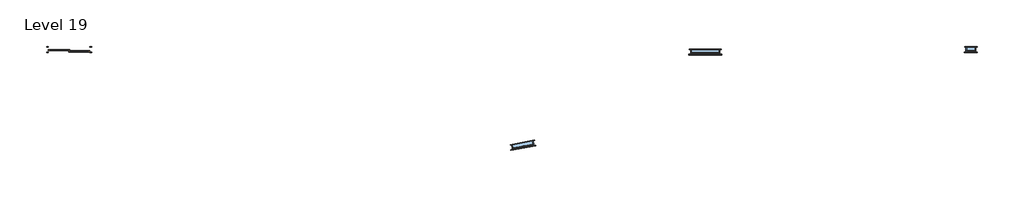
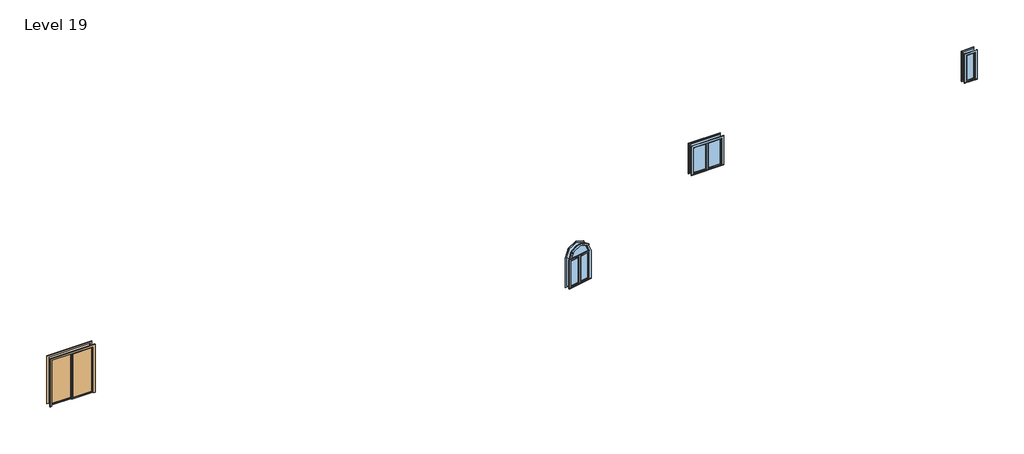
# One storey: 3 windows, 1 door.
"""IFC4 building model written with IfcOpenShell, lengths in millimetres."""

from ifc_helpers import new_model, si_unit, origin, place, context, project, spatial, transform, mapped, element, save
from components import door_076b30e0, window_cf4adaea, window_a765b88f, window_0862ab64

model = new_model("IFC4")

# Units and contexts
model_context = context("Model", 3, world=origin())
ifc_project = project(units=[si_unit("LENGTHUNIT", "METRE", prefix="MILLI")], contexts=[model_context])

# Site, building, storey
site = spatial("IfcSite", under=ifc_project)
building = spatial("IfcBuilding", under=site)
storey = spatial("IfcBuildingStorey", under=building, Name="Level 19", Elevation=32918.4)

# Door
placement = place(None, origin())
door_shape = door_076b30e0(model_context)
element("IfcDoor", 1, ObjectType="Door-Double-Sliding : 68\" x 80\"", at=placement, inside=storey, context=model_context, shape_type="MappedRepresentation", body=[
    mapped(door_shape, transform((-16521.785279, -12227.7237084, 32918.4), x_axis=(-1.0, 0.0, 0.0), y_axis=(0.0, -1.0, 0.0), z_axis=(0.0, 0.0, 1.0))),
])

# Windows
window_shape = window_cf4adaea(model_context)
element("IfcWindow", 2, ObjectType="36\" x 48\"", at=placement, inside=storey, context=model_context, shape_type="MappedRepresentation", body=[
    mapped(window_shape, transform((2348.7105307, -16344.9215105, 32918.4), x_axis=(-0.9830283621128597, -0.1834536434135567, 0.0), y_axis=(0.1834536434135567, -0.9830283621128597, 0.0), z_axis=(0.0, 0.0, 1.0))),
])
window_2_shape = window_a765b88f(model_context)
element("IfcWindow", 3, ObjectType="Awning with Trim : 16\" x 48\"", at=placement, inside=storey, context=model_context, shape_type="MappedRepresentation", body=[
    mapped(window_2_shape, transform((20968.614721, -12354.7237084, 32918.4), x_axis=(-1.0, 0.0, 0.0), y_axis=(0.0, -1.0, 0.0), z_axis=(0.0, 0.0, 1.0))),
])
window_3_shape = window_0862ab64(model_context)
element("IfcWindow", 4, ObjectType="Casement Dbl with Trim : 48\" x 48\"", at=placement, inside=storey, context=model_context, shape_type="MappedRepresentation", body=[
    mapped(window_3_shape, transform((9924.3594464, -12437.2737084, 32918.4), x_axis=(-1.0, 0.0, 0.0), y_axis=(0.0, -1.0, 0.0), z_axis=(0.0, 0.0, 1.0))),
])

save(model, "model.ifc")

# Revit data of these elements
# Type "Door-Double-Sliding : 68\" x 80\""
#   Type Mark = "10"
#   Construction Type Id = "opn-d45"
#   Assembly Code = "C1020"
#   Analytic Construction = "Wood frame, double glass door "
#   Thickness = 0' - 2"
#   Thermal Resistance (R) = 1.8150 (h·ft²·°F)/BTU
#   Heat Transfer Coefficient (U) = 0.5510 BTU/(h·ft²·°F)
#   Height = 6' - 8"
#   Rail Width = 0' - 2"
#   Stiles = 0' - 2"
#   Trim Projection Ext = 0' - 1"
#   Trim Projection Int = 0' - 1"
#   Trim Width = 0' - 3"
#   Width = 5' - 8"
#   Define Thermal Properties by = 1
#   Glazing = Glass
#   Panel Material = Wood - Birch - Solid Stained Light Low Gloss
#   Trim Material = Paint - Sienna
#   Visual Light Transmittance = 0
#   Solar Heat Gain Coefficient = 0
#   Function = (empty or 0)
#   Wall Closure = (empty or 0)
# Type "36\" x 48\""
#   Type Mark = "38"
#   Construction Type Id = "SGL"
#   Assembly Code = "B2020100"
#   Analytic Construction = "Large single-glazed windows"
#   Visual Light Transmittance = 0.9
#   Solar Heat Gain Coefficient = 0.86
#   Heat Transfer Coefficient (U) = 0.979472 BTU/(h·ft²·°F)
#   Height = 4' - 0"
#   Default Sill Height = 3' - 0"
#   Trim Projection - Ext. = 0' - 0 1/2"
#   Trim Projection - Int. = 0' - 0 3/4"
#   Trim Width - Exterior = 0' - 3 1/2"
#   Trim Width - Interior = 0' - 3 1/2"
#   Width = 3' - 0"
#   Window Inset = 0' - 0 3/4"
#   Define Thermal Properties by = 1
#   Glass Pane Material = Glass
#   Sash Material = Sash
#   Trim Exterior Material = Trim
#   Trim Interior Material = Trim
#   Wall Closure = (empty or 0)
# Type "Awning with Trim : 16\" x 48\""
#   Type Mark = "14"
#   Construction Type Id = "GSP4R"
#   Assembly Code = "B2020100"
#   Analytic Construction = "1/8 in Pilkington single glazing"
#   Visual Light Transmittance = 0.9
#   Solar Heat Gain Coefficient = 0.78
#   Heat Transfer Coefficient (U) = 0.6496 BTU/(h·ft²·°F)
#   Height = 4' - 0"
#   Default Sill Height = 3' - 0"
#   Trim Projection - Ext. = 0' - 0 1/2"
#   Trim Projection - Int. = 0' - 0 3/4"
#   Trim Width - Exterior = 0' - 3 1/2"
#   Trim Width - Interior = 0' - 3 1/2"
#   Width = 1' - 4"
#   Window Inset = 0' - 0 3/4"
#   Define Thermal Properties by = 1
#   Glass Pane Material = Glass
#   Sash Material = Sash
#   Trim Exterior Material = Trim
#   Trim Interior Material = Trim
#   Wall Closure = (empty or 0)
# Type "Casement Dbl with Trim : 48\" x 48\""
#   Type Mark = "34"
#   Construction Type Id = "GSP4R"
#   Assembly Code = "B2020100"
#   Analytic Construction = "1/8 in Pilkington single glazing"
#   Visual Light Transmittance = 0.9
#   Solar Heat Gain Coefficient = 0.78
#   Heat Transfer Coefficient (U) = 0.6496 BTU/(h·ft²·°F)
#   Height = 4' - 0"
#   Default Sill Height = 3' - 0"
#   Trim Projection - Ext. = 0' - 0 1/2"
#   Trim Projection - Int. = 0' - 0 3/4"
#   Trim Width - Exterior = 0' - 3 1/2"
#   Trim Width - Interior = 0' - 3 1/2"
#   Width = 4' - 0"
#   Window Inset = 0' - 0 3/4"
#   Define Thermal Properties by = 1
#   Glass Pane Material = Glass
#   Sash Material = Sash
#   Trim Exterior Material = Trim
#   Trim Interior Material = Trim
#   Wall Closure = (empty or 0)
# Element 1 (IfcDoor, "Door-Double-Sliding : 68\" x 80\"")
#   Phase Created = New Construction
#   Materials on its faces: "Paint - Sienna", "Wood - Birch - Solid Stained Light Low Gloss", "Glass"
# Element 2 (IfcWindow, "36\" x 48\"")
#   Mark = "24"
#   Phase Created = New Construction
#   Materials on its faces: "Sash", "Trim", "Glass"
# Element 3 (IfcWindow, "Awning with Trim : 16\" x 48\"")
#   Mark = "58"
#   Phase Created = New Construction
#   Materials on its faces: "Sash", "Trim", "Glass"
# Element 4 (IfcWindow, "Casement Dbl with Trim : 48\" x 48\"")
#   Mark = "7"
#   Phase Created = New Construction
#   Materials on its faces: "Sash", "Trim", "Glass"
# Materials
#   "Glass": class "Glass", colour RGB 0 128 192, transparency 0.75, Description = "Soda Lime Glass", Cost = 0
#   "Wood - Birch - Solid Stained Light Low Gloss": class "Wood", colour RGB 210 159 95, transparency 0, Cost = 0
#   "Paint - Sienna": colour RGB 118 70 51, transparency 0, Cost = 0
#   "Sash": class "Wood", colour RGB 224 178 126, transparency 0
#   "Trim": class "Wood", colour RGB 224 178 126, transparency 0
